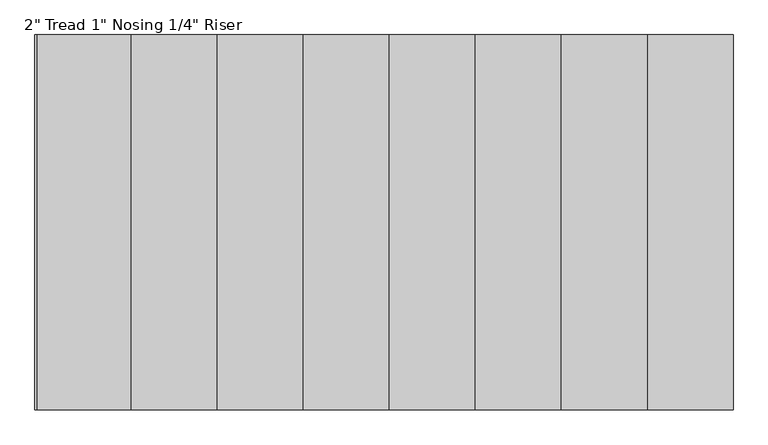
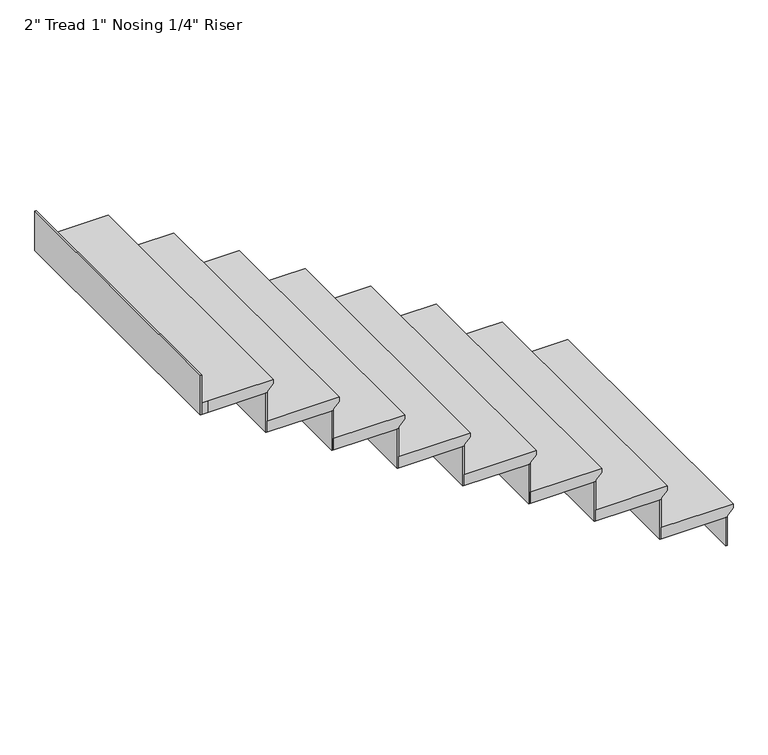
"""IFC4 building model written with IfcOpenShell, lengths in millimetres: stair flight geometry."""

from ifc_helpers import new_model, si_unit, origin, place, context, project, spatial, faceted_brep, source, transform, mapped, element, save


def stair_flight_969e3d78(model_context):
    return source(origin(), model_context, "Body", "Brep", [
        faceted_brep([(-5888.8791271, 6233.3953048, 158.75), (-5888.8791271, 6233.3953048, 177.8), (-5888.8791271, 5014.1953048, 177.8), (-5888.8791271, 5014.1953048, 158.75), (-5914.2791271, 6233.3953048, 133.35), (-5914.2791271, 5014.1953048, 133.35), (-6193.6791271, 6233.3953048, 177.8), (-6193.6791271, 5014.1953048, 177.8), (-5914.2791271, 5014.1953048, 127.0), (-6193.6791271, 5014.1953048, 127.0), (-6193.6791271, 6233.3953048, 127.0), (-5914.2791271, 6233.3953048, 127.0)], [[[0, 1, 2, 3]], [[4, 0, 3, 5]], [[2, 1, 6, 7]], [[8, 9, 10, 11]], [[2, 7, 9, 8, 5, 3]], [[8, 11, 4, 5]], [[6, 1, 0, 4, 11, 10]], [[7, 6, 10, 9]]]),
        faceted_brep([(-5914.2791271, 6233.3953048, 127.0), (-5914.2791271, 6233.3953048, 0.0), (-5920.6291271, 6233.3953048, 0.0), (-5920.6291271, 6233.3953048, 127.0), (-5914.2791271, 5014.1953048, 127.0), (-5920.6291271, 5014.1953048, 127.0), (-5920.6291271, 5014.1953048, 0.0), (-5914.2791271, 5014.1953048, 0.0)], [[[0, 1, 2, 3]], [[4, 5, 6, 7]], [[1, 0, 4, 7]], [[2, 1, 7, 6]], [[3, 2, 6, 5]], [[0, 3, 5, 4]]]),
        faceted_brep([(-6193.6791271, 6233.3953048, 304.8), (-6193.6791271, 6233.3953048, 127.0), (-6200.0291271, 6233.3953048, 127.0), (-6200.0291271, 6233.3953048, 304.8), (-6193.6791271, 5014.1953048, 304.8), (-6200.0291271, 5014.1953048, 304.8), (-6200.0291271, 5014.1953048, 127.0), (-6193.6791271, 5014.1953048, 127.0)], [[[0, 1, 2, 3]], [[4, 5, 6, 7]], [[1, 0, 4, 7]], [[2, 1, 7, 6]], [[3, 2, 6, 5]], [[0, 3, 5, 4]]]),
        faceted_brep([(-6168.2791271, 5014.1953048, 355.6), (-6168.2791271, 6233.3953048, 355.6), (-6473.0791271, 6233.3953048, 355.6), (-6473.0791271, 5014.1953048, 355.6), (-6193.6791271, 5014.1953048, 304.8), (-6473.0791271, 5014.1953048, 304.8), (-6473.0791271, 6233.3953048, 304.8), (-6193.6791271, 6233.3953048, 304.8), (-6193.6791271, 5014.1953048, 311.15), (-6168.2791271, 5014.1953048, 336.55), (-6193.6791271, 6233.3953048, 311.15), (-6168.2791271, 6233.3953048, 336.55)], [[[0, 1, 2, 3]], [[4, 5, 6, 7]], [[0, 3, 5, 4, 8, 9]], [[4, 7, 10, 8]], [[2, 1, 11, 10, 7, 6]], [[3, 2, 6, 5]], [[11, 1, 0, 9]], [[10, 11, 9, 8]]]),
        faceted_brep([(-6473.0791271, 6233.3953048, 482.6), (-6473.0791271, 6233.3953048, 304.8), (-6479.4291271, 6233.3953048, 304.8), (-6479.4291271, 6233.3953048, 482.6), (-6473.0791271, 5014.1953048, 482.6), (-6479.4291271, 5014.1953048, 482.6), (-6479.4291271, 5014.1953048, 304.8), (-6473.0791271, 5014.1953048, 304.8)], [[[0, 1, 2, 3]], [[4, 5, 6, 7]], [[1, 0, 4, 7]], [[2, 1, 7, 6]], [[3, 2, 6, 5]], [[0, 3, 5, 4]]]),
        faceted_brep([(-6447.6791271, 5014.1953048, 533.4), (-6447.6791271, 6233.3953048, 533.4), (-6752.4791271, 6233.3953048, 533.4), (-6752.4791271, 5014.1953048, 533.4), (-6473.0791271, 5014.1953048, 482.6), (-6752.4791271, 5014.1953048, 482.6), (-6752.4791271, 6233.3953048, 482.6), (-6473.0791271, 6233.3953048, 482.6), (-6473.0791271, 5014.1953048, 488.95), (-6447.6791271, 5014.1953048, 514.35), (-6473.0791271, 6233.3953048, 488.95), (-6447.6791271, 6233.3953048, 514.35)], [[[0, 1, 2, 3]], [[4, 5, 6, 7]], [[0, 3, 5, 4, 8, 9]], [[4, 7, 10, 8]], [[2, 1, 11, 10, 7, 6]], [[3, 2, 6, 5]], [[11, 1, 0, 9]], [[10, 11, 9, 8]]]),
        faceted_brep([(-6752.4791271, 6233.3953048, 660.4), (-6752.4791271, 6233.3953048, 482.6), (-6758.8291271, 6233.3953048, 482.6), (-6758.8291271, 6233.3953048, 660.4), (-6752.4791271, 5014.1953048, 660.4), (-6758.8291271, 5014.1953048, 660.4), (-6758.8291271, 5014.1953048, 482.6), (-6752.4791271, 5014.1953048, 482.6)], [[[0, 1, 2, 3]], [[4, 5, 6, 7]], [[1, 0, 4, 7]], [[2, 1, 7, 6]], [[3, 2, 6, 5]], [[0, 3, 5, 4]]]),
        faceted_brep([(-6727.0791271, 5014.1953048, 711.2), (-6727.0791271, 6233.3953048, 711.2), (-7031.8791271, 6233.3953048, 711.2), (-7031.8791271, 5014.1953048, 711.2), (-6752.4791271, 5014.1953048, 660.4), (-7031.8791271, 5014.1953048, 660.4), (-7031.8791271, 6233.3953048, 660.4), (-6752.4791271, 6233.3953048, 660.4), (-6752.4791271, 5014.1953048, 666.75), (-6727.0791271, 5014.1953048, 692.15), (-6752.4791271, 6233.3953048, 666.75), (-6727.0791271, 6233.3953048, 692.15)], [[[0, 1, 2, 3]], [[4, 5, 6, 7]], [[0, 3, 5, 4, 8, 9]], [[4, 7, 10, 8]], [[2, 1, 11, 10, 7, 6]], [[3, 2, 6, 5]], [[11, 1, 0, 9]], [[10, 11, 9, 8]]]),
        faceted_brep([(-7031.8791271, 6233.3953048, 838.2), (-7031.8791271, 6233.3953048, 660.4), (-7038.2291271, 6233.3953048, 660.4), (-7038.2291271, 6233.3953048, 838.2), (-7031.8791271, 5014.1953048, 838.2), (-7038.2291271, 5014.1953048, 838.2), (-7038.2291271, 5014.1953048, 660.4), (-7031.8791271, 5014.1953048, 660.4)], [[[0, 1, 2, 3]], [[4, 5, 6, 7]], [[1, 0, 4, 7]], [[2, 1, 7, 6]], [[3, 2, 6, 5]], [[0, 3, 5, 4]]]),
        faceted_brep([(-7006.4791271, 5014.1953048, 889.0), (-7006.4791271, 6233.3953048, 889.0), (-7311.2791271, 6233.3953048, 889.0), (-7311.2791271, 5014.1953048, 889.0), (-7031.8791271, 5014.1953048, 838.2), (-7311.2791271, 5014.1953048, 838.2), (-7311.2791271, 6233.3953048, 838.2), (-7031.8791271, 6233.3953048, 838.2), (-7031.8791271, 5014.1953048, 844.55), (-7006.4791271, 5014.1953048, 869.95), (-7031.8791271, 6233.3953048, 844.55), (-7006.4791271, 6233.3953048, 869.95)], [[[0, 1, 2, 3]], [[4, 5, 6, 7]], [[0, 3, 5, 4, 8, 9]], [[4, 7, 10, 8]], [[2, 1, 11, 10, 7, 6]], [[3, 2, 6, 5]], [[11, 1, 0, 9]], [[10, 11, 9, 8]]]),
        faceted_brep([(-7311.2791271, 6233.3953048, 1016.0), (-7311.2791271, 6233.3953048, 838.2), (-7317.6291271, 6233.3953048, 838.2), (-7317.6291271, 6233.3953048, 1016.0), (-7311.2791271, 5014.1953048, 1016.0), (-7317.6291271, 5014.1953048, 1016.0), (-7317.6291271, 5014.1953048, 838.2), (-7311.2791271, 5014.1953048, 838.2)], [[[0, 1, 2, 3]], [[4, 5, 6, 7]], [[1, 0, 4, 7]], [[2, 1, 7, 6]], [[3, 2, 6, 5]], [[0, 3, 5, 4]]]),
        faceted_brep([(-7285.8791271, 5014.1953048, 1066.8), (-7285.8791271, 6233.3953048, 1066.8), (-7590.6791271, 6233.3953048, 1066.8), (-7590.6791271, 5014.1953048, 1066.8), (-7311.2791271, 5014.1953048, 1016.0), (-7590.6791271, 5014.1953048, 1016.0), (-7590.6791271, 6233.3953048, 1016.0), (-7311.2791271, 6233.3953048, 1016.0), (-7311.2791271, 5014.1953048, 1022.35), (-7285.8791271, 5014.1953048, 1047.75), (-7311.2791271, 6233.3953048, 1022.35), (-7285.8791271, 6233.3953048, 1047.75)], [[[0, 1, 2, 3]], [[4, 5, 6, 7]], [[0, 3, 5, 4, 8, 9]], [[4, 7, 10, 8]], [[2, 1, 11, 10, 7, 6]], [[3, 2, 6, 5]], [[11, 1, 0, 9]], [[10, 11, 9, 8]]]),
        faceted_brep([(-7590.6791271, 6233.3953048, 1193.8), (-7590.6791271, 6233.3953048, 1016.0), (-7597.0291271, 6233.3953048, 1016.0), (-7597.0291271, 6233.3953048, 1193.8), (-7590.6791271, 5014.1953048, 1193.8), (-7597.0291271, 5014.1953048, 1193.8), (-7597.0291271, 5014.1953048, 1016.0), (-7590.6791271, 5014.1953048, 1016.0)], [[[0, 1, 2, 3]], [[4, 5, 6, 7]], [[1, 0, 4, 7]], [[2, 1, 7, 6]], [[3, 2, 6, 5]], [[0, 3, 5, 4]]]),
        faceted_brep([(-7565.2791271, 5014.1953048, 1244.6), (-7565.2791271, 6233.3953048, 1244.6), (-7870.0791271, 6233.3953048, 1244.6), (-7870.0791271, 5014.1953048, 1244.6), (-7590.6791271, 5014.1953048, 1193.8), (-7870.0791271, 5014.1953048, 1193.8), (-7870.0791271, 6233.3953048, 1193.8), (-7590.6791271, 6233.3953048, 1193.8), (-7590.6791271, 5014.1953048, 1200.15), (-7565.2791271, 5014.1953048, 1225.55), (-7590.6791271, 6233.3953048, 1200.15), (-7565.2791271, 6233.3953048, 1225.55)], [[[0, 1, 2, 3]], [[4, 5, 6, 7]], [[0, 3, 5, 4, 8, 9]], [[4, 7, 10, 8]], [[2, 1, 11, 10, 7, 6]], [[3, 2, 6, 5]], [[11, 1, 0, 9]], [[10, 11, 9, 8]]]),
        faceted_brep([(-8149.4791271, 6233.3953048, 1549.4), (-8149.4791271, 6233.3953048, 1371.6), (-8155.8291271, 6233.3953048, 1371.6), (-8155.8291271, 6233.3953048, 1549.4), (-8149.4791271, 5014.1953048, 1549.4), (-8155.8291271, 5014.1953048, 1549.4), (-8155.8291271, 5014.1953048, 1371.6), (-8149.4791271, 5014.1953048, 1371.6)], [[[0, 1, 2, 3]], [[4, 5, 6, 7]], [[1, 0, 4, 7]], [[2, 1, 7, 6]], [[3, 2, 6, 5]], [[0, 3, 5, 4]]]),
        faceted_brep([(-7870.0791271, 6233.3953048, 1371.6), (-7870.0791271, 6233.3953048, 1193.8), (-7876.4291271, 6233.3953048, 1193.8), (-7876.4291271, 6233.3953048, 1371.6), (-7870.0791271, 5014.1953048, 1371.6), (-7876.4291271, 5014.1953048, 1371.6), (-7876.4291271, 5014.1953048, 1193.8), (-7870.0791271, 5014.1953048, 1193.8)], [[[0, 1, 2, 3]], [[4, 5, 6, 7]], [[1, 0, 4, 7]], [[2, 1, 7, 6]], [[3, 2, 6, 5]], [[0, 3, 5, 4]]]),
        faceted_brep([(-8149.4791271, 5014.1953048, 1422.4), (-8124.0791271, 5014.1953048, 1422.4), (-7844.6791271, 5014.1953048, 1422.4), (-7844.6791271, 6233.3953048, 1422.4), (-8149.4791271, 6233.3953048, 1422.4), (-8124.0791271, 5014.1953048, 1371.6), (-8149.4791271, 5014.1953048, 1371.6), (-8149.4791271, 6233.3953048, 1371.6), (-7870.0791271, 6233.3953048, 1371.6), (-7870.0791271, 5014.1953048, 1371.6), (-7870.0791271, 5014.1953048, 1377.95), (-7844.6791271, 5014.1953048, 1403.35), (-7870.0791271, 6233.3953048, 1377.95), (-7844.6791271, 6233.3953048, 1403.35)], [[[0, 1, 2, 3, 4]], [[5, 6, 7, 8, 9]], [[1, 0, 6, 5]], [[2, 1, 5, 9, 10, 11]], [[9, 8, 12, 10]], [[4, 3, 13, 12, 8, 7]], [[0, 4, 7, 6]], [[13, 3, 2, 11]], [[12, 13, 11, 10]]]),
    ])


if __name__ == "__main__":
    model = new_model("IFC4")
    model_context = context("Model", 3, world=origin())
    ifc_project = project(units=[si_unit("LENGTHUNIT", "METRE", prefix="MILLI")], contexts=[model_context])
    site = spatial("IfcSite", under=ifc_project)
    building = spatial("IfcBuilding", under=site)
    placement = place(None, origin())
    stair_flight_shape = stair_flight_969e3d78(model_context)
    element("IfcStairFlight", 1, ObjectType="2\" Tread 1\" Nosing 1/4\" Riser", at=placement, inside=building, context=model_context, shape_type="MappedRepresentation", body=[
        mapped(stair_flight_shape, transform((0.0, 0.0, 0.0), x_axis=(1.0, 0.0, 0.0), y_axis=(0.0, 1.0, 0.0), z_axis=(0.0, 0.0, 1.0))),
    ])
    save(model, "model.ifc")
